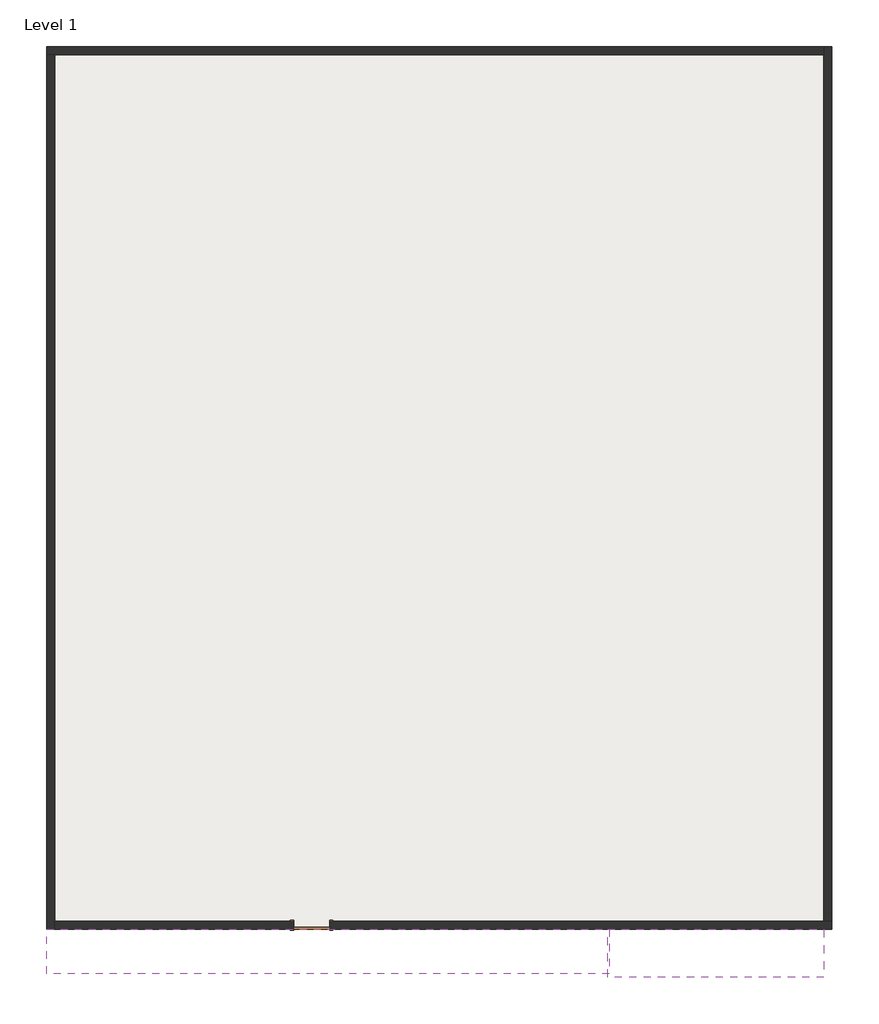
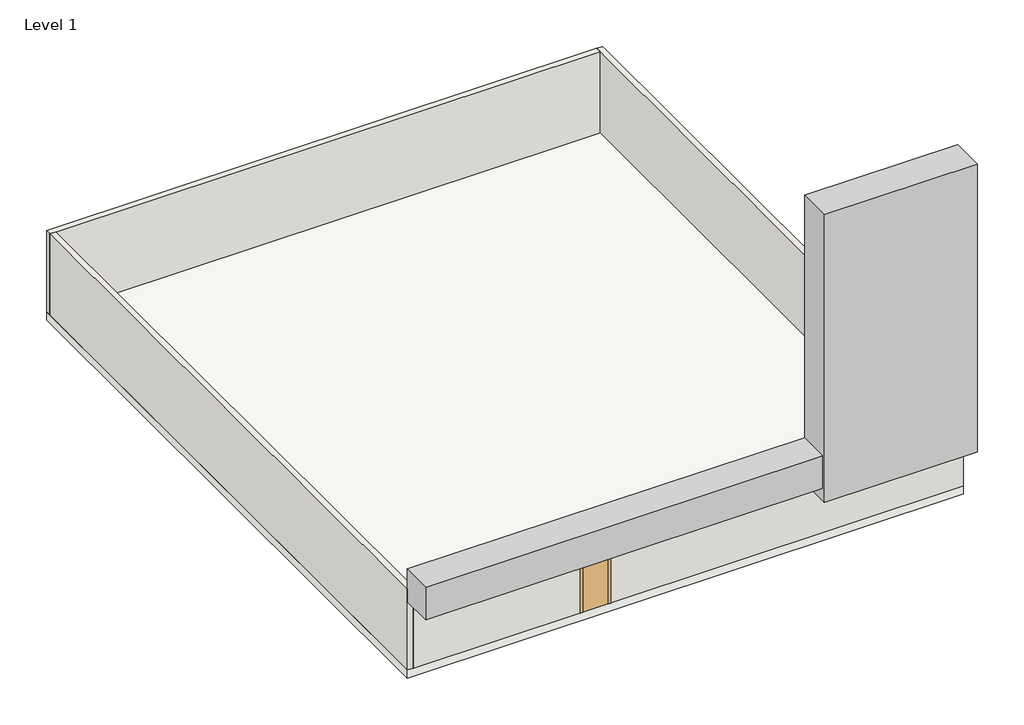
# One storey: 4 walls, 2 proxies, 1 door, 1 slab.
"""IFC4 building model written with IfcOpenShell, lengths in millimetres."""

from ifc_helpers import new_model, si_unit, frame, origin, place, context, project, spatial, polyline, outline, extrude, faceted_brep, transform, mapped, element, save
from components import generic_models_1_generic_models_1_a4a6df41, generic_models_6_generic_models_6_03283b1a, door_54dd4da4

model = new_model("IFC4")

# Units and contexts
model_context = context("Model", 3, world=origin())
ifc_project = project(units=[si_unit("LENGTHUNIT", "METRE", prefix="MILLI")], contexts=[model_context])

# Site, building, storey
site = spatial("IfcSite", under=ifc_project)
building = spatial("IfcBuilding", under=site)
storey = spatial("IfcBuildingStorey", under=building, Name="Level 1", Elevation=0.0)

# Proxies
placement = place(None, origin())
generic_models_1_generic_models_1_shape = generic_models_1_generic_models_1_a4a6df41(model_context)
element("IfcBuildingElementProxy", 1, Name="Generic Models 1 : Generic Models 1", ObjectType="Generic Models 1 : Generic Models 1", at=placement, inside=storey, context=model_context, shape_type="MappedRepresentation", body=[
    mapped(generic_models_1_generic_models_1_shape, transform((0.0, 0.0, 0.0), x_axis=(1.0, 0.0, 0.0), y_axis=(0.0, 1.0, 0.0), z_axis=(0.0, 0.0, 1.0))),
])
generic_models_6_generic_models_6_shape = generic_models_6_generic_models_6_03283b1a(model_context)
element("IfcBuildingElementProxy", 2, Name="Generic Models 6 : Generic Models 6", ObjectType="Generic Models 6 : Generic Models 6", at=placement, inside=storey, context=model_context, shape_type="MappedRepresentation", body=[
    mapped(generic_models_6_generic_models_6_shape, transform((0.0, 0.0, 0.0), x_axis=(1.0, 0.0, 0.0), y_axis=(0.0, 1.0, 0.0), z_axis=(0.0, 0.0, 1.0))),
])

# Door
door_shape = door_54dd4da4(model_context)
element("IfcDoor", 3, ObjectType="Single-Flush : 36\" x 84\"", at=placement, inside=storey, context=model_context, shape_type="MappedRepresentation", body=[
    mapped(door_shape, transform((-3304.3625896, -8539.5821053, 0.0), x_axis=(-1.0, 0.0, 0.0), y_axis=(0.0, -1.0, 0.0), z_axis=(0.0, 0.0, 1.0))),
])

# Slab
element("IfcSlab", 4, ObjectType="Generic - 12\"", at=placement, inside=storey, context=model_context, shape_type="SweptSolid", body=[
    extrude(outline(polyline([(9751.2374104, 13507.6178947), (9751.2374104, -8641.1821053), (-9959.1625896, -8641.1821053), (-9959.1625896, 13507.6178947), (9751.2374104, 13507.6178947)])), frame((0.0, 0.0, -304.8), z_axis=(0.0, 0.0, 1.0), x_axis=(1.0, 0.0, 0.0)), (0.0, 0.0, 1.0), 304.8),
])

# Walls
element("IfcWall", 5, ObjectType="Generic - 8\"", at=placement, inside=storey, context=model_context, shape_type="Brep", body=[
    faceted_brep([(-9959.1625896, 13304.4178947, 0.0), (-9755.9625896, 13304.4178947, 0.0), (9548.0374104, 13304.4178947, 0.0), (9548.0374104, 13304.4178947, 3048.0), (-9755.9625896, 13304.4178947, 3048.0), (-9959.1625896, 13304.4178947, 3048.0), (-9959.1625896, 13507.6178947, 0.0), (-9959.1625896, 13507.6178947, 3048.0), (9548.0374104, 13507.6178947, 3048.0), (9548.0374104, 13507.6178947, 0.0)], [[[0, 1, 2, 3, 4, 5]], [[6, 7, 8, 9]], [[2, 1, 0, 6, 9]], [[0, 5, 7, 6]], [[3, 2, 9, 8]], [[5, 4, 3, 8, 7]]]),
])
element("IfcWall", 6, ObjectType="Generic - 8\"", at=placement, inside=storey, context=model_context, shape_type="Brep", body=[
    faceted_brep([(-9755.9625896, -8641.1821053, 0.0), (-9755.9625896, -8437.9821053, 0.0), (-9755.9625896, 13304.4178947, 0.0), (-9755.9625896, 13304.4178947, 3048.0), (-9755.9625896, -8437.9821053, 3048.0), (-9755.9625896, -8641.1821053, 3048.0), (-9959.1625896, -8641.1821053, 0.0), (-9959.1625896, -8641.1821053, 3048.0), (-9959.1625896, 13304.4178947, 3048.0), (-9959.1625896, 13304.4178947, 0.0)], [[[0, 1, 2, 3, 4, 5]], [[6, 7, 8, 9]], [[2, 1, 0, 6, 9]], [[0, 5, 7, 6]], [[3, 2, 9, 8]], [[5, 4, 3, 8, 7]]]),
])
element("IfcWall", 7, ObjectType="Generic - 8\"", at=placement, inside=storey, context=model_context, shape_type="Brep", body=[
    faceted_brep([(-3761.5625896, -8437.9821053, 2133.6), (-3761.5625896, -8437.9821053, 0.0), (-9755.9625896, -8437.9821053, 0.0), (-9755.9625896, -8437.9821053, 3048.0), (9548.0374104, -8437.9821053, 3048.0), (9751.2374104, -8437.9821053, 3048.0), (9751.2374104, -8437.9821053, 0.0), (9548.0374104, -8437.9821053, 0.0), (-2847.1625896, -8437.9821053, 0.0), (-2847.1625896, -8437.9821053, 2133.6), (-9755.9625896, -8641.1821053, 0.0), (-3761.5625896, -8641.1821053, 0.0), (-3761.5625896, -8641.1821053, 2133.6), (-2847.1625896, -8641.1821053, 2133.6), (-2847.1625896, -8641.1821053, 0.0), (9751.2374104, -8641.1821053, 0.0), (9751.2374104, -8641.1821053, 3048.0), (-9755.9625896, -8641.1821053, 3048.0)], [[[0, 1, 2, 3, 4, 5, 6, 7, 8, 9]], [[10, 11, 12, 13, 14, 15, 16, 17]], [[2, 1, 11, 10]], [[8, 7, 6, 15, 14]], [[6, 5, 16, 15]], [[3, 2, 10, 17]], [[5, 4, 3, 17, 16]], [[12, 11, 1, 0]], [[13, 12, 0, 9]], [[14, 13, 9, 8]]]),
])
element("IfcWall", 8, ObjectType="Generic - 8\"", at=placement, inside=storey, context=model_context, shape_type="Brep", body=[
    faceted_brep([(9548.0374104, 13507.6178947, 0.0), (9548.0374104, 13304.4178947, 0.0), (9548.0374104, -8437.9821053, 0.0), (9548.0374104, -8437.9821053, 3048.0), (9548.0374104, 13304.4178947, 3048.0), (9548.0374104, 13507.6178947, 3048.0), (9751.2374104, 13507.6178947, 0.0), (9751.2374104, 13507.6178947, 3048.0), (9751.2374104, -8437.9821053, 3048.0), (9751.2374104, -8437.9821053, 0.0)], [[[0, 1, 2, 3, 4, 5]], [[6, 7, 8, 9]], [[2, 1, 0, 6, 9]], [[0, 5, 7, 6]], [[3, 2, 9, 8]], [[5, 4, 3, 8, 7]]]),
])

save(model, "model.ifc")

# Revit data of these elements
# Type "Single-Flush : 36\" x 84\""
#   Type Mark = "1"
#   Construction Type Id = "MDOOR"
#   Assembly Code = "C1020"
#   Analytic Construction = "Metal"
#   Thickness = 0' - 2"
#   Heat Transfer Coefficient (U) = 0.651978 BTU/(h·ft²·°F)
#   Height = 7' - 0"
#   Trim Projection Ext = 0' - 1"
#   Trim Projection Int = 0' - 1"
#   Trim Width = 0' - 3"
#   Width = 3' - 0"
#   Define Thermal Properties by = 1
#   Door Material = Door - Panel
#   Frame Material = Door - Frame
#   Visual Light Transmittance = 0
#   Solar Heat Gain Coefficient = 0
#   Function = (empty or 0)
#   Wall Closure = (empty or 0)
# Type "Generic - 12\""
#   Assembly Code = "B1010"
#   Function = 0
#   Layers, outside or top first: 1' - 0" no material (function 1)
# Type "Generic - 8\""
#   Assembly Code = "B2010"
#   Layers, outside or top first: 0' - 8" no material (function 1)
# Element 1 (IfcBuildingElementProxy, "Generic Models 1 : Generic Models 1")
#   Phase Created = New Construction
# Element 2 (IfcBuildingElementProxy, "Generic Models 6 : Generic Models 6")
#   Phase Created = New Construction
# Element 3 (IfcDoor, "Single-Flush : 36\" x 84\"")
#   Phase Created = New Construction
#   Materials on its faces: "Door - Frame", "Door - Panel"
# Element 4 (IfcSlab, "Generic - 12\"")
#   Height Offset From Level = 0' - 0"
#   Phase Created = New Construction
#   Materials on its faces: "Default Floor"
# Element 5 (IfcWall, "Generic - 8\"")
#   Top Offset = 0' - 0"
#   Base Offset = 0' - 0"
#   Unconnected Height = 30' - 0.34115"
#   wall height = 30' - 0.34115"
#   Phase Created = New Construction
#   Base Constraint = Level 1
#   Materials on its faces: "Default Wall"
# Elements 6, 7, 8 (IfcWall, "Generic - 8\"")
#   Top Offset = 0' - 0"
#   Base Offset = 0' - 0"
#   Unconnected Height = 30' - 0"
#   wall height = 30' - 0"
#   Phase Created = New Construction
#   Base Constraint = Level 1
#   Materials on its faces: "Default Wall"
# Materials
#   "Door - Panel": class "Wood", colour RGB 210 159 95, transparency 0
#   "Door - Frame": colour RGB 118 70 51, transparency 0
#   "Default Floor": colour RGB 128 128 128, transparency 0
#   "Default Wall": colour RGB 128 128 128, transparency 0
